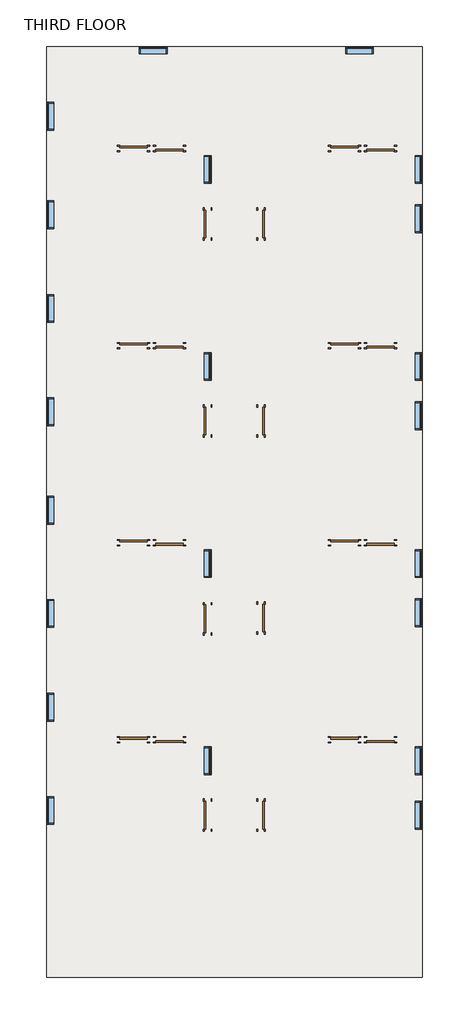
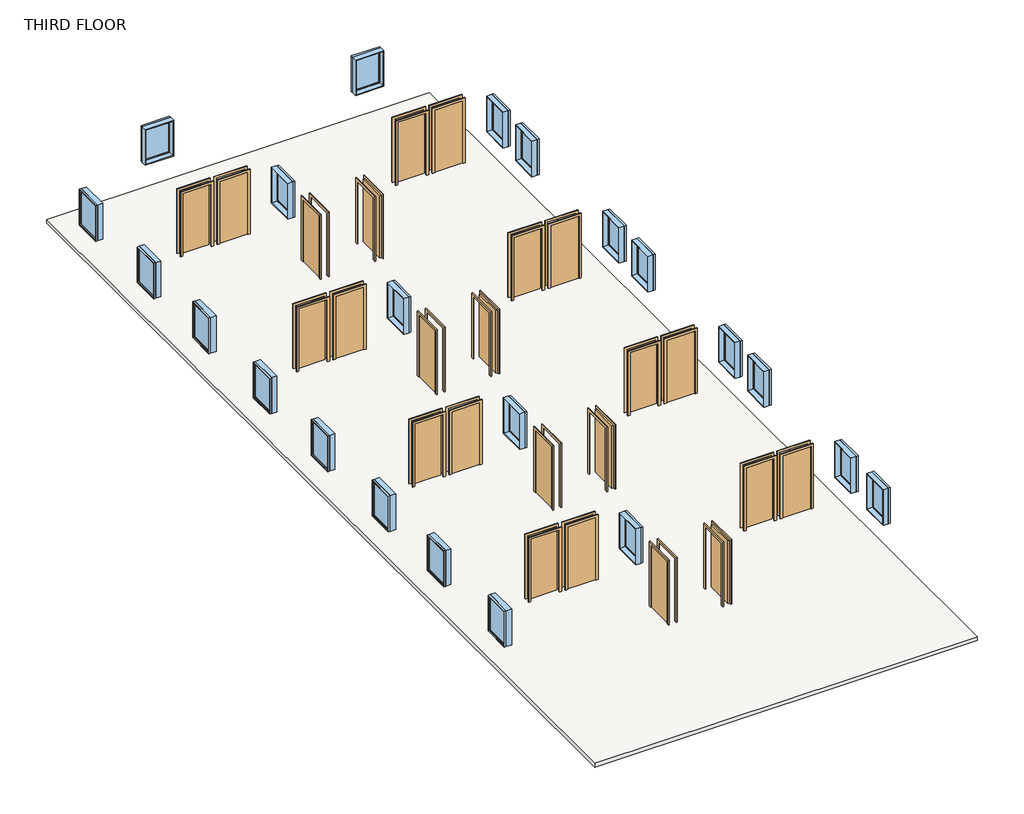
# One storey: 24 doors, 22 windows, 1 slab.
"""IFC4 building model written with IfcOpenShell, lengths in millimetres."""

from ifc_helpers import new_model, si_unit, frame, origin, place, context, project, spatial, polyline, outline, extrude, transform, mapped, element, save
from components import door_686f89d2, door_16372e1c, door_a90ba1ad, door_0ca8825f, window_c1f32544

model = new_model("IFC4")

# Units and contexts
model_context = context("Model", 3, world=origin())
ifc_project = project(units=[si_unit("LENGTHUNIT", "METRE", prefix="MILLI")], contexts=[model_context])

# Site, building, storey
site = spatial("IfcSite", under=ifc_project)
building = spatial("IfcBuilding", under=site)
storey = spatial("IfcBuildingStorey", under=building, Name="THIRD FLOOR", Elevation=9601.2)

# Doors
placement = place(None, origin())
door_shape = door_686f89d2(model_context)
element("IfcDoor", 1, ObjectType="Single-Flush : 36\" x 84\"", at=placement, inside=storey, context=model_context, shape_type="MappedRepresentation", body=[
    mapped(door_shape, transform((-9863.5902461, 11952.2710592, 9601.2), x_axis=(-1.0, 0.0, 0.0), y_axis=(0.0, -1.0, 0.0), z_axis=(0.0, 0.0, 1.0))),
])
element("IfcDoor", 2, ObjectType="Single-Flush : 36\" x 84\"", at=placement, inside=storey, context=model_context, shape_type="MappedRepresentation", body=[
    mapped(door_shape, transform((-2929.3902461, 11952.2710592, 9601.2), x_axis=(-1.0, 0.0, 0.0), y_axis=(0.0, -1.0, 0.0), z_axis=(0.0, 0.0, 1.0))),
])
element("IfcDoor", 3, ObjectType="Single-Flush : 36\" x 84\"", at=placement, inside=storey, context=model_context, shape_type="MappedRepresentation", body=[
    mapped(door_shape, transform((-9863.5902461, 5475.2710592, 9601.2), x_axis=(-1.0, 0.0, 0.0), y_axis=(0.0, -1.0, 0.0), z_axis=(0.0, 0.0, 1.0))),
])
element("IfcDoor", 4, ObjectType="Single-Flush : 36\" x 84\"", at=placement, inside=storey, context=model_context, shape_type="MappedRepresentation", body=[
    mapped(door_shape, transform((-9863.5902461, -1001.7289408, 9601.2), x_axis=(-1.0, 0.0, 0.0), y_axis=(0.0, -1.0, 0.0), z_axis=(0.0, 0.0, 1.0))),
])
element("IfcDoor", 5, ObjectType="Single-Flush : 36\" x 84\"", at=placement, inside=storey, context=model_context, shape_type="MappedRepresentation", body=[
    mapped(door_shape, transform((-9863.5902461, -7478.7289408, 9601.2), x_axis=(-1.0, 0.0, 0.0), y_axis=(0.0, -1.0, 0.0), z_axis=(0.0, 0.0, 1.0))),
])
element("IfcDoor", 6, ObjectType="Single-Flush : 36\" x 84\"", at=placement, inside=storey, context=model_context, shape_type="MappedRepresentation", body=[
    mapped(door_shape, transform((-2929.3902461, 5475.2710592, 9601.2), x_axis=(-1.0, 0.0, 0.0), y_axis=(0.0, -1.0, 0.0), z_axis=(0.0, 0.0, 1.0))),
])
element("IfcDoor", 7, ObjectType="Single-Flush : 36\" x 84\"", at=placement, inside=storey, context=model_context, shape_type="MappedRepresentation", body=[
    mapped(door_shape, transform((-2929.3902461, -1001.7289408, 9601.2), x_axis=(-1.0, 0.0, 0.0), y_axis=(0.0, -1.0, 0.0), z_axis=(0.0, 0.0, 1.0))),
])
element("IfcDoor", 8, ObjectType="Single-Flush : 36\" x 84\"", at=placement, inside=storey, context=model_context, shape_type="MappedRepresentation", body=[
    mapped(door_shape, transform((-2929.3902461, -7478.7289408, 9601.2), x_axis=(-1.0, 0.0, 0.0), y_axis=(0.0, -1.0, 0.0), z_axis=(0.0, 0.0, 1.0))),
])
door_2_shape = door_16372e1c(model_context)
element("IfcDoor", 9, ObjectType="Single-Flush : 36\" x 84\"", at=placement, inside=storey, context=model_context, shape_type="MappedRepresentation", body=[
    mapped(door_2_shape, transform((-8682.4902461, 11952.2710592, 9601.2), x_axis=(-1.0, 0.0, 0.0), y_axis=(0.0, -1.0, 0.0), z_axis=(0.0, 0.0, 1.0))),
])
element("IfcDoor", 10, ObjectType="Single-Flush : 36\" x 84\"", at=placement, inside=storey, context=model_context, shape_type="MappedRepresentation", body=[
    mapped(door_2_shape, transform((-1748.2902461, 11952.2710592, 9601.2), x_axis=(-1.0, 0.0, 0.0), y_axis=(0.0, -1.0, 0.0), z_axis=(0.0, 0.0, 1.0))),
])
element("IfcDoor", 11, ObjectType="Single-Flush : 36\" x 84\"", at=placement, inside=storey, context=model_context, shape_type="MappedRepresentation", body=[
    mapped(door_2_shape, transform((-8682.4902461, 5475.2710592, 9601.2), x_axis=(-1.0, 0.0, 0.0), y_axis=(0.0, -1.0, 0.0), z_axis=(0.0, 0.0, 1.0))),
])
element("IfcDoor", 12, ObjectType="Single-Flush : 36\" x 84\"", at=placement, inside=storey, context=model_context, shape_type="MappedRepresentation", body=[
    mapped(door_2_shape, transform((-8682.4902461, -1001.7289408, 9601.2), x_axis=(-1.0, 0.0, 0.0), y_axis=(0.0, -1.0, 0.0), z_axis=(0.0, 0.0, 1.0))),
])
element("IfcDoor", 13, ObjectType="Single-Flush : 36\" x 84\"", at=placement, inside=storey, context=model_context, shape_type="MappedRepresentation", body=[
    mapped(door_2_shape, transform((-8682.4902461, -7478.7289408, 9601.2), x_axis=(-1.0, 0.0, 0.0), y_axis=(0.0, -1.0, 0.0), z_axis=(0.0, 0.0, 1.0))),
])
element("IfcDoor", 14, ObjectType="Single-Flush : 36\" x 84\"", at=placement, inside=storey, context=model_context, shape_type="MappedRepresentation", body=[
    mapped(door_2_shape, transform((-1748.2902461, 5475.2710592, 9601.2), x_axis=(-1.0, 0.0, 0.0), y_axis=(0.0, -1.0, 0.0), z_axis=(0.0, 0.0, 1.0))),
])
element("IfcDoor", 15, ObjectType="Single-Flush : 36\" x 84\"", at=placement, inside=storey, context=model_context, shape_type="MappedRepresentation", body=[
    mapped(door_2_shape, transform((-1748.2902461, -1001.7289408, 9601.2), x_axis=(-1.0, 0.0, 0.0), y_axis=(0.0, -1.0, 0.0), z_axis=(0.0, 0.0, 1.0))),
])
element("IfcDoor", 16, ObjectType="Single-Flush : 36\" x 84\"", at=placement, inside=storey, context=model_context, shape_type="MappedRepresentation", body=[
    mapped(door_2_shape, transform((-1748.2902461, -7478.7289408, 9601.2), x_axis=(-1.0, 0.0, 0.0), y_axis=(0.0, -1.0, 0.0), z_axis=(0.0, 0.0, 1.0))),
])
door_3_shape = door_a90ba1ad(model_context)
element("IfcDoor", 17, ObjectType="Single-Flush : 36\" x 84\"", at=placement, inside=storey, context=model_context, shape_type="MappedRepresentation", body=[
    mapped(door_3_shape, transform((-7425.1902461, 9475.7710592, 9601.2), x_axis=(0.0, -1.0, 0.0), y_axis=(1.0, 0.0, 0.0), z_axis=(0.0, 0.0, 1.0))),
])
element("IfcDoor", 18, ObjectType="Single-Flush : 36\" x 84\"", at=placement, inside=storey, context=model_context, shape_type="MappedRepresentation", body=[
    mapped(door_3_shape, transform((-7425.1902461, 2998.7710592, 9601.2), x_axis=(0.0, -1.0, 0.0), y_axis=(1.0, 0.0, 0.0), z_axis=(0.0, 0.0, 1.0))),
])
element("IfcDoor", 19, ObjectType="Single-Flush : 36\" x 84\"", at=placement, inside=storey, context=model_context, shape_type="MappedRepresentation", body=[
    mapped(door_3_shape, transform((-7425.1902461, -3503.6289408, 9601.2), x_axis=(0.0, -1.0, 0.0), y_axis=(1.0, 0.0, 0.0), z_axis=(0.0, 0.0, 1.0))),
])
element("IfcDoor", 20, ObjectType="Single-Flush : 36\" x 84\"", at=placement, inside=storey, context=model_context, shape_type="MappedRepresentation", body=[
    mapped(door_3_shape, transform((-7425.1902461, -9955.2289408, 9601.2), x_axis=(0.0, -1.0, 0.0), y_axis=(1.0, 0.0, 0.0), z_axis=(0.0, 0.0, 1.0))),
])
door_4_shape = door_0ca8825f(model_context)
element("IfcDoor", 21, ObjectType="Single-Flush : 36\" x 84\"", at=placement, inside=storey, context=model_context, shape_type="MappedRepresentation", body=[
    mapped(door_4_shape, transform((-5672.5902461, 9475.7710592, 9601.2), x_axis=(0.0, -1.0, 0.0), y_axis=(1.0, 0.0, 0.0), z_axis=(0.0, 0.0, 1.0))),
])
element("IfcDoor", 22, ObjectType="Single-Flush : 36\" x 84\"", at=placement, inside=storey, context=model_context, shape_type="MappedRepresentation", body=[
    mapped(door_4_shape, transform((-5672.5902461, 2998.7710592, 9601.2), x_axis=(0.0, -1.0, 0.0), y_axis=(1.0, 0.0, 0.0), z_axis=(0.0, 0.0, 1.0))),
])
element("IfcDoor", 23, ObjectType="Single-Flush : 36\" x 84\"", at=placement, inside=storey, context=model_context, shape_type="MappedRepresentation", body=[
    mapped(door_4_shape, transform((-5672.5902461, -3478.2289408, 9601.2), x_axis=(0.0, -1.0, 0.0), y_axis=(1.0, 0.0, 0.0), z_axis=(0.0, 0.0, 1.0))),
])
element("IfcDoor", 24, ObjectType="Single-Flush : 36\" x 84\"", at=placement, inside=storey, context=model_context, shape_type="MappedRepresentation", body=[
    mapped(door_4_shape, transform((-5672.5902461, -9955.2289408, 9601.2), x_axis=(0.0, -1.0, 0.0), y_axis=(1.0, 0.0, 0.0), z_axis=(0.0, 0.0, 1.0))),
])

# Slab
element("IfcSlab", 25, ObjectType="Generic - 12\"", at=placement, inside=storey, context=model_context, shape_type="SweptSolid", body=[
    extrude(outline(polyline([(-376.6902461, 15305.0710592), (-376.6902461, -15289.2289408), (-12721.0902461, -15289.2289408), (-12721.0902461, 15305.0710592), (-376.6902461, 15305.0710592)])), frame((0.0, 0.0, 9474.2), z_axis=(0.0, 0.0, 1.0), x_axis=(1.0, 0.0, 0.0)), (0.0, 0.0, 1.0), 127.0),
])

# Windows
window_shape = window_c1f32544(model_context)
element("IfcWindow", 26, ObjectType="Fixed : 36\" x 48\"", at=placement, inside=storey, context=model_context, shape_type="MappedRepresentation", body=[
    mapped(window_shape, transform((-490.9902461, 4751.3710592, 9601.2), x_axis=(0.0, -1.0, 0.0), y_axis=(1.0, 0.0, 0.0), z_axis=(0.0, 0.0, 1.0))),
])
element("IfcWindow", 27, ObjectType="Fixed : 36\" x 48\"", at=placement, inside=storey, context=model_context, shape_type="MappedRepresentation", body=[
    mapped(window_shape, transform((-490.9902461, 3132.1210592, 9601.2), x_axis=(0.0, -1.0, 0.0), y_axis=(1.0, 0.0, 0.0), z_axis=(0.0, 0.0, 1.0))),
])
element("IfcWindow", 28, ObjectType="Fixed : 36\" x 48\"", at=placement, inside=storey, context=model_context, shape_type="MappedRepresentation", body=[
    mapped(window_shape, transform((-490.9902461, -1725.6289408, 9601.2), x_axis=(0.0, -1.0, 0.0), y_axis=(1.0, 0.0, 0.0), z_axis=(0.0, 0.0, 1.0))),
])
element("IfcWindow", 29, ObjectType="Fixed : 36\" x 48\"", at=placement, inside=storey, context=model_context, shape_type="MappedRepresentation", body=[
    mapped(window_shape, transform((-490.9902461, -3344.8789408, 9601.2), x_axis=(0.0, -1.0, 0.0), y_axis=(1.0, 0.0, 0.0), z_axis=(0.0, 0.0, 1.0))),
])
element("IfcWindow", 30, ObjectType="Fixed : 36\" x 48\"", at=placement, inside=storey, context=model_context, shape_type="MappedRepresentation", body=[
    mapped(window_shape, transform((-490.9902461, -8202.6289408, 9601.2), x_axis=(0.0, -1.0, 0.0), y_axis=(1.0, 0.0, 0.0), z_axis=(0.0, 0.0, 1.0))),
])
element("IfcWindow", 31, ObjectType="Fixed : 36\" x 48\"", at=placement, inside=storey, context=model_context, shape_type="MappedRepresentation", body=[
    mapped(window_shape, transform((-490.9902461, -9993.3289408, 9601.2), x_axis=(0.0, -1.0, 0.0), y_axis=(1.0, 0.0, 0.0), z_axis=(0.0, 0.0, 1.0))),
])
element("IfcWindow", 32, ObjectType="Fixed : 36\" x 48\"", at=placement, inside=storey, context=model_context, shape_type="MappedRepresentation", body=[
    mapped(window_shape, transform((-490.9902461, 9609.1210592, 9601.2), x_axis=(0.0, -1.0, 0.0), y_axis=(1.0, 0.0, 0.0), z_axis=(0.0, 0.0, 1.0))),
])
element("IfcWindow", 33, ObjectType="Fixed : 36\" x 48\"", at=placement, inside=storey, context=model_context, shape_type="MappedRepresentation", body=[
    mapped(window_shape, transform((-490.9902461, 11228.3710592, 9601.2), x_axis=(0.0, -1.0, 0.0), y_axis=(1.0, 0.0, 0.0), z_axis=(0.0, 0.0, 1.0))),
])
element("IfcWindow", 34, ObjectType="Fixed : 36\" x 48\"", at=placement, inside=storey, context=model_context, shape_type="MappedRepresentation", body=[
    mapped(window_shape, transform((-2395.9902461, 15190.7710592, 9601.2), x_axis=(1.0, 0.0, 0.0), y_axis=(0.0, 1.0, 0.0), z_axis=(0.0, 0.0, 1.0))),
])
element("IfcWindow", 35, ObjectType="Fixed : 36\" x 48\"", at=placement, inside=storey, context=model_context, shape_type="MappedRepresentation", body=[
    mapped(window_shape, transform((-9177.7902461, 15190.7710592, 9601.2), x_axis=(1.0, 0.0, 0.0), y_axis=(0.0, 1.0, 0.0), z_axis=(0.0, 0.0, 1.0))),
])
element("IfcWindow", 36, ObjectType="Fixed : 36\" x 48\"", at=placement, inside=storey, context=model_context, shape_type="MappedRepresentation", body=[
    mapped(window_shape, transform((-12606.7902461, 13057.1710592, 9601.2), x_axis=(0.0, 1.0, 0.0), y_axis=(-1.0, 0.0, 0.0), z_axis=(0.0, 0.0, 1.0))),
])
element("IfcWindow", 37, ObjectType="Fixed : 36\" x 48\"", at=placement, inside=storey, context=model_context, shape_type="MappedRepresentation", body=[
    mapped(window_shape, transform((-12606.7902461, 9818.6710592, 9601.2), x_axis=(0.0, 1.0, 0.0), y_axis=(-1.0, 0.0, 0.0), z_axis=(0.0, 0.0, 1.0))),
])
element("IfcWindow", 38, ObjectType="Fixed : 36\" x 48\"", at=placement, inside=storey, context=model_context, shape_type="MappedRepresentation", body=[
    mapped(window_shape, transform((-12606.7902461, 6732.5710592, 9601.2), x_axis=(0.0, 1.0, 0.0), y_axis=(-1.0, 0.0, 0.0), z_axis=(0.0, 0.0, 1.0))),
])
element("IfcWindow", 39, ObjectType="Fixed : 36\" x 48\"", at=placement, inside=storey, context=model_context, shape_type="MappedRepresentation", body=[
    mapped(window_shape, transform((-12606.7902461, 3341.6710592, 9601.2), x_axis=(0.0, 1.0, 0.0), y_axis=(-1.0, 0.0, 0.0), z_axis=(0.0, 0.0, 1.0))),
])
element("IfcWindow", 40, ObjectType="Fixed : 36\" x 48\"", at=placement, inside=storey, context=model_context, shape_type="MappedRepresentation", body=[
    mapped(window_shape, transform((-12606.7902461, 103.1710592, 9601.2), x_axis=(0.0, 1.0, 0.0), y_axis=(-1.0, 0.0, 0.0), z_axis=(0.0, 0.0, 1.0))),
])
element("IfcWindow", 41, ObjectType="Fixed : 36\" x 48\"", at=placement, inside=storey, context=model_context, shape_type="MappedRepresentation", body=[
    mapped(window_shape, transform((-12606.7902461, -3287.7289408, 9601.2), x_axis=(0.0, 1.0, 0.0), y_axis=(-1.0, 0.0, 0.0), z_axis=(0.0, 0.0, 1.0))),
])
element("IfcWindow", 42, ObjectType="Fixed : 36\" x 48\"", at=placement, inside=storey, context=model_context, shape_type="MappedRepresentation", body=[
    mapped(window_shape, transform((-12606.7902461, -6373.8289408, 9601.2), x_axis=(0.0, 1.0, 0.0), y_axis=(-1.0, 0.0, 0.0), z_axis=(0.0, 0.0, 1.0))),
])
element("IfcWindow", 43, ObjectType="Fixed : 36\" x 48\"", at=placement, inside=storey, context=model_context, shape_type="MappedRepresentation", body=[
    mapped(window_shape, transform((-12606.7902461, -9764.7289408, 9601.2), x_axis=(0.0, 1.0, 0.0), y_axis=(-1.0, 0.0, 0.0), z_axis=(0.0, 0.0, 1.0))),
])
element("IfcWindow", 44, ObjectType="Fixed : 36\" x 48\"", at=placement, inside=storey, context=model_context, shape_type="MappedRepresentation", body=[
    mapped(window_shape, transform((-7425.1902461, -1725.6289408, 9601.2), x_axis=(0.0, -1.0, 0.0), y_axis=(1.0, 0.0, 0.0), z_axis=(0.0, 0.0, 1.0))),
])
element("IfcWindow", 45, ObjectType="Fixed : 36\" x 48\"", at=placement, inside=storey, context=model_context, shape_type="MappedRepresentation", body=[
    mapped(window_shape, transform((-7425.1902461, 4751.3710592, 9601.2), x_axis=(0.0, -1.0, 0.0), y_axis=(1.0, 0.0, 0.0), z_axis=(0.0, 0.0, 1.0))),
])
element("IfcWindow", 46, ObjectType="Fixed : 36\" x 48\"", at=placement, inside=storey, context=model_context, shape_type="MappedRepresentation", body=[
    mapped(window_shape, transform((-7425.1902461, 11228.3710592, 9601.2), x_axis=(0.0, -1.0, 0.0), y_axis=(1.0, 0.0, 0.0), z_axis=(0.0, 0.0, 1.0))),
])
element("IfcWindow", 47, ObjectType="Fixed : 36\" x 48\"", at=placement, inside=storey, context=model_context, shape_type="MappedRepresentation", body=[
    mapped(window_shape, transform((-7425.1902461, -8202.6289408, 9601.2), x_axis=(0.0, -1.0, 0.0), y_axis=(1.0, 0.0, 0.0), z_axis=(0.0, 0.0, 1.0))),
])

save(model, "model.ifc")

# Revit data of these elements
# Type "Single-Flush : 36\" x 84\""
#   Type Mark = "1"
#   Construction Type Id = "MDOOR"
#   Assembly Code = "C1020"
#   Analytic Construction = "Metal"
#   Thickness = 0' - 2"
#   Heat Transfer Coefficient (U) = 0.651978 BTU/(h·ft²·°F)
#   Height = 7' - 0"
#   Trim Projection Ext = 0' - 1"
#   Trim Projection Int = 0' - 1"
#   Trim Width = 0' - 3"
#   Width = 3' - 0"
#   Define Thermal Properties by = 1
#   Door Material = Door - Panel
#   Frame Material = Door - Frame
#   Visual Light Transmittance = 0
#   Solar Heat Gain Coefficient = 0
#   Function = (empty or 0)
#   Wall Closure = (empty or 0)
# Type "Generic - 12\""
#   Assembly Code = "B1010"
#   Function = 0
#   Layers, outside or top first: 0' - 5" no material (function 1)
# Type "Fixed : 36\" x 48\""
#   Type Mark = "1"
#   Construction Type Id = "GSP4R"
#   Assembly Code = "B2020100"
#   Analytic Construction = "1/8 in Pilkington single glazing"
#   Visual Light Transmittance = 0.9
#   Solar Heat Gain Coefficient = 0.78
#   Heat Transfer Coefficient (U) = 0.6496 BTU/(h·ft²·°F)
#   Height = 4' - 0"
#   Default Sill Height = 3' - 0"
#   Width = 3' - 0"
#   Window Inset = 0' - 0 3/4"
#   Define Thermal Properties by = 1
#   Glass Pane Material = Glass
#   Sash Material = Sash
#   Wall Closure = (empty or 0)
# Elements 1, 2, 3, 4, 5, 6, 7, 8, 9, 10, 11, 12, 13, 14, 15, 16, 17, 18, 19, 20, 21, 22, 23, 24 (IfcDoor, "Single-Flush : 36\" x 84\"")
#   Phase Created = New Construction
#   Materials on its faces: "Door - Frame", "Door - Panel"
# Element 25 (IfcSlab, "Generic - 12\"")
#   Height Offset From Level = 0' - 0"
#   Phase Created = New Construction
#   Materials on its faces: "Default Floor"
# Element 26 (IfcWindow, "Fixed : 36\" x 48\"")
#   Mark = "71"
#   Phase Created = New Construction
#   Materials on its faces: "Sash", "Glass"
# Element 27 (IfcWindow, "Fixed : 36\" x 48\"")
#   Mark = "72"
#   Phase Created = New Construction
#   Materials on its faces: "Sash", "Glass"
# Element 28 (IfcWindow, "Fixed : 36\" x 48\"")
#   Mark = "73"
#   Phase Created = New Construction
#   Materials on its faces: "Sash", "Glass"
# Element 29 (IfcWindow, "Fixed : 36\" x 48\"")
#   Mark = "74"
#   Phase Created = New Construction
#   Materials on its faces: "Sash", "Glass"
# Element 30 (IfcWindow, "Fixed : 36\" x 48\"")
#   Mark = "75"
#   Phase Created = New Construction
#   Materials on its faces: "Sash", "Glass"
# Element 31 (IfcWindow, "Fixed : 36\" x 48\"")
#   Mark = "76"
#   Phase Created = New Construction
#   Materials on its faces: "Sash", "Glass"
# Element 32 (IfcWindow, "Fixed : 36\" x 48\"")
#   Mark = "77"
#   Phase Created = New Construction
#   Materials on its faces: "Sash", "Glass"
# Element 33 (IfcWindow, "Fixed : 36\" x 48\"")
#   Mark = "78"
#   Phase Created = New Construction
#   Materials on its faces: "Sash", "Glass"
# Element 34 (IfcWindow, "Fixed : 36\" x 48\"")
#   Mark = "79"
#   Phase Created = New Construction
#   Materials on its faces: "Sash", "Glass"
# Element 35 (IfcWindow, "Fixed : 36\" x 48\"")
#   Mark = "80"
#   Phase Created = New Construction
#   Materials on its faces: "Sash", "Glass"
# Element 36 (IfcWindow, "Fixed : 36\" x 48\"")
#   Mark = "81"
#   Phase Created = New Construction
#   Materials on its faces: "Sash", "Glass"
# Element 37 (IfcWindow, "Fixed : 36\" x 48\"")
#   Mark = "82"
#   Phase Created = New Construction
#   Materials on its faces: "Sash", "Glass"
# Element 38 (IfcWindow, "Fixed : 36\" x 48\"")
#   Mark = "83"
#   Phase Created = New Construction
#   Materials on its faces: "Sash", "Glass"
# Element 39 (IfcWindow, "Fixed : 36\" x 48\"")
#   Mark = "84"
#   Phase Created = New Construction
#   Materials on its faces: "Sash", "Glass"
# Element 40 (IfcWindow, "Fixed : 36\" x 48\"")
#   Mark = "85"
#   Phase Created = New Construction
#   Materials on its faces: "Sash", "Glass"
# Element 41 (IfcWindow, "Fixed : 36\" x 48\"")
#   Mark = "86"
#   Phase Created = New Construction
#   Materials on its faces: "Sash", "Glass"
# Element 42 (IfcWindow, "Fixed : 36\" x 48\"")
#   Mark = "87"
#   Phase Created = New Construction
#   Materials on its faces: "Sash", "Glass"
# Element 43 (IfcWindow, "Fixed : 36\" x 48\"")
#   Mark = "88"
#   Phase Created = New Construction
#   Materials on its faces: "Sash", "Glass"
# Element 44 (IfcWindow, "Fixed : 36\" x 48\"")
#   Mark = "89"
#   Phase Created = New Construction
#   Materials on its faces: "Sash", "Glass"
# Element 45 (IfcWindow, "Fixed : 36\" x 48\"")
#   Mark = "90"
#   Phase Created = New Construction
#   Materials on its faces: "Sash", "Glass"
# Element 46 (IfcWindow, "Fixed : 36\" x 48\"")
#   Mark = "91"
#   Phase Created = New Construction
#   Materials on its faces: "Sash", "Glass"
# Element 47 (IfcWindow, "Fixed : 36\" x 48\"")
#   Mark = "92"
#   Phase Created = New Construction
#   Materials on its faces: "Sash", "Glass"
# Materials
#   "Door - Panel": class "Wood", colour RGB 210 159 95, transparency 0
#   "Door - Frame": colour RGB 118 70 51, transparency 0
#   "Glass": class "Glass", colour RGB 0 128 192, transparency 0.75, Description = "Soda Lime Glass", Cost = 0
#   "Sash": class "Wood", colour RGB 224 178 126, transparency 0
#   "Default Floor": colour RGB 128 128 128, transparency 0
